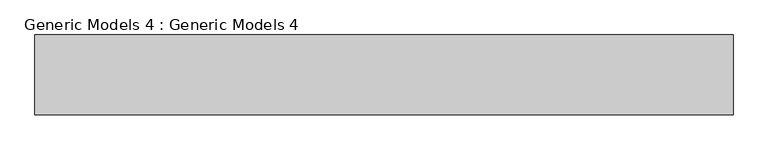
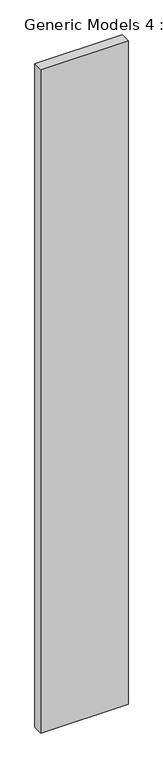
"""IFC4 building model written with IfcOpenShell, lengths in millimetres: proxy geometry, Generic Models 4 : Generic Models 4."""

from ifc_helpers import new_model, si_unit, frame, origin, place, context, project, spatial, polyline, outline, extrude, source, transform, mapped, element, save


def generic_models_4_generic_models_4_e8bbcad5(model_context):
    return source(origin(), model_context, "Body", "SweptSolid", [
        extrude(outline(polyline([(-14180.7645284, -9552.8468404), (-15512.0003513, -9552.8468404), (-15512.0003513, -9400.4468404), (-14180.7645284, -9400.4468404), (-14180.7645284, -9552.8468404)])), frame((0.0, 0.0, 304.8), z_axis=(0.0, 0.0, 1.0), x_axis=(1.0, 0.0, 0.0)), (0.0, 0.0, 1.0), 10684.0045332),
    ])


if __name__ == "__main__":
    model = new_model("IFC4")
    model_context = context("Model", 3, world=origin())
    ifc_project = project(units=[si_unit("LENGTHUNIT", "METRE", prefix="MILLI")], contexts=[model_context])
    site = spatial("IfcSite", under=ifc_project)
    building = spatial("IfcBuilding", under=site)
    placement = place(None, origin())
    generic_models_4_generic_models_4_shape = generic_models_4_generic_models_4_e8bbcad5(model_context)
    element("IfcBuildingElementProxy", 1, Name="Generic Models 4 : Generic Models 4", ObjectType="Generic Models 4 : Generic Models 4", at=placement, inside=building, context=model_context, shape_type="MappedRepresentation", body=[
        mapped(generic_models_4_generic_models_4_shape, transform((0.0, 0.0, 0.0), x_axis=(1.0, 0.0, 0.0), y_axis=(0.0, 1.0, 0.0), z_axis=(0.0, 0.0, 1.0))),
    ])
    save(model, "model.ifc")
